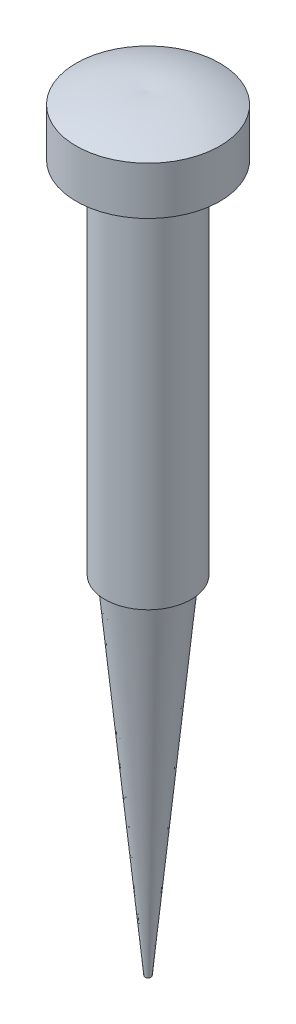
from build123d import *

# Parameters (mm, degrees)
TIP_BASE_CIRCLE_3_R      = 1.5
TAPERED_NEEDLE_TIP_DEPTH = 14.5
TAPERED_NEEDLE_TIP_TAPER = 5.42


with BuildPart() as part:
    # Head and Stem Profile → Head and Stem Revolve (revolve)
    with BuildSketch(Plane.XY, mode=Mode.PRIVATE) as head_and_stem_revolve_sk:
        with BuildLine():
            Line((0, 0), (0, 17.5))
            ThreePointArc((0, 17.5), (1.532206849, 17.443241097), (3, 17))
            Line((3, 17), (3, 15))
            Line((3, 15), (1.8, 15))
            Line((1.8, 15), (1.8, 0))
            Line((1.8, 0), (0, 0))
        make_face()
    revolve(head_and_stem_revolve_sk.sketch.rotate(Axis((0, 0, 0), (0, 1, 0)), 90), axis=Axis((0, 0, 0), (0, 1, 0)))

    # Tip Base Circle Ø3 → Tapered Needle Tip (add)
    with BuildSketch(Plane.XZ):
        Circle(TIP_BASE_CIRCLE_3_R)
    extrude(amount=TAPERED_NEEDLE_TIP_DEPTH, taper=TAPERED_NEEDLE_TIP_TAPER)


solid = part.part
